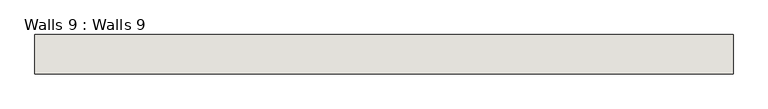
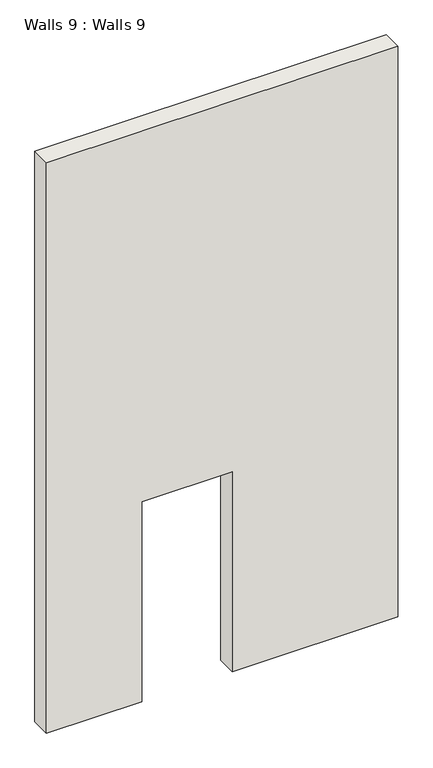
"""IFC4 building model written with IfcOpenShell, lengths in millimetres: wall geometry, Walls 9 : Walls 9."""

from ifc_helpers import new_model, si_unit, frame, origin, place, context, project, spatial, polyline, outline, extrude, source, transform, mapped, element, save


def walls_9_walls_9_f00b2fad(model_context):
    return source(origin(), model_context, "Body", "SweptSolid", [
        extrude(outline(polyline([(6096.0, -9784.4289001), (6096.0, -13337.2289001), (0.0, -13337.2289001), (0.0, -12374.1283679), (2134.0, -12374.1283679), (2134.0, -11459.1283679), (0.0, -11459.1283679), (0.0, -9784.4289001), (6096.0, -9784.4289001)])), frame((0.0, -3390.9180898, 0.0), z_axis=(0.0, 1.0, 0.0), x_axis=(0.0, 0.0, 1.0)), (0.0, 0.0, 1.0), 200.0),
    ])


if __name__ == "__main__":
    model = new_model("IFC4")
    model_context = context("Model", 3, world=origin())
    ifc_project = project(units=[si_unit("LENGTHUNIT", "METRE", prefix="MILLI")], contexts=[model_context])
    site = spatial("IfcSite", under=ifc_project)
    building = spatial("IfcBuilding", under=site)
    placement = place(None, origin())
    walls_9_walls_9_shape = walls_9_walls_9_f00b2fad(model_context)
    element("IfcWall", 1, ObjectType="Walls 9 : Walls 9", at=placement, inside=building, context=model_context, shape_type="MappedRepresentation", body=[
        mapped(walls_9_walls_9_shape, transform((0.0, 0.0, 0.0), x_axis=(1.0, 0.0, 0.0), y_axis=(0.0, 1.0, 0.0), z_axis=(0.0, 0.0, 1.0))),
    ])
    save(model, "model.ifc")

# Revit data of these elements
# Element 1 (IfcWall, "Walls 9 : Walls 9")
#   Materials on its faces: "Default Wall"
# Materials
#   "Default Wall": colour RGB 80 80 80, transparency 0
